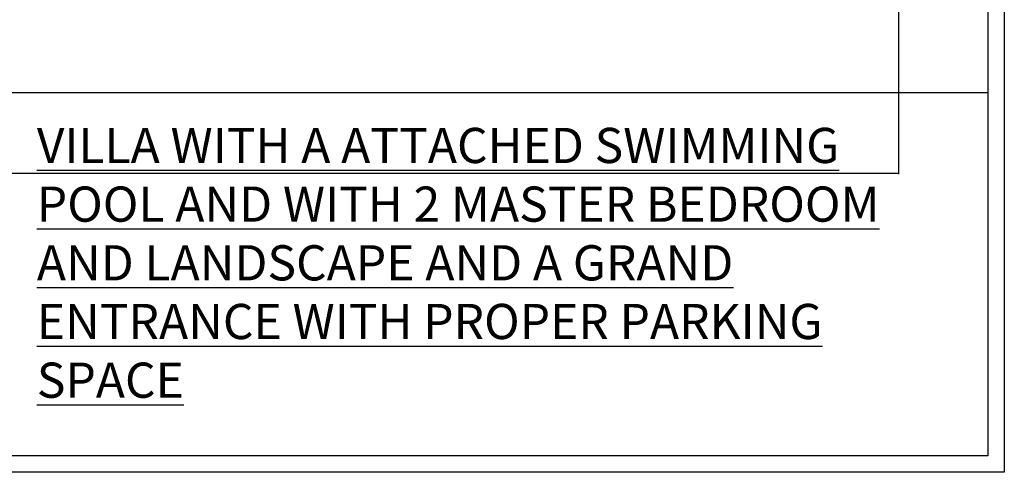
# Model space of a CAD drawing. Units: inches. Extents: x 84 to 1044, y -280 to 906.
# Tile 22 of 105: x 700 to 1027, y -280 to -129. Entities that reach past the tile are written whole.
import ezdxf

# ---------------------------------------------------------------- set-up
doc = ezdxf.new("R2010")
doc.units = ezdxf.units.IN
doc.layers.add('A-ANNO-DIMS', color=2, linetype='Continuous', lineweight=18)
doc.layers.add('A-ANNO-TTLB', color=7, linetype='Continuous', lineweight=25)
doc.styles.add('1-100DIM', font='txt', dxfattribs={"height": 0.3})
doc.styles.get("Standard").update_dxf_attribs({"font": 'arial.ttf'})
doc.dimstyles.get("Standard").update_dxf_attribs({"dimtxt": 0.18, "dimasz": 0.18, "dimexe": 0.18, "dimexo": 0.0625, "dimgap": 0.09, "dimtad": 0, "dimtih": 1, "dimtoh": 1, "dimdec": 4, "dimzin": 0, "dimdsep": 46, "dimtxsty": 'Standard', "dimcen": 0.09, "dimadec": 0, "dimazin": 0, "dimtfac": 1, "dimtdec": 4, "dimtofl": 0, "dimtmove": 0, "dimatfit": 3, "dimfxl": 1, "dimtolj": 1, "dimtzin": 0, "dimarcsym": 0})

# ---------------------------------------------------------------- blocks, each defined once
blk = doc.blocks.new('*D60')
at = {"layer": 'A-ANNO-DIMS', "color": 0, "lineweight": -2, "transparency": 16777216}
for p, q in [((134.18, -121.94), (134.18, -180.64)), ((992.07, -121.94), (992.07, -180.64)), ((134.36, -180.46), (562.73, -180.46)), ((991.89, -180.46), (563.52, -180.46))]:
    blk.add_line(p, q, dxfattribs=at)
at = {"layer": 'A-ANNO-DIMS', "color": 0, "transparency": 16777216}
for points in [[(134.36, -180.43), (134.36, -180.49), (134.18, -180.46)], [(991.89, -180.43), (991.89, -180.49), (992.07, -180.46)]]:
    blk.add_solid(points, dxfattribs=at)
at = {"layer": 'Defpoints', "color": 0, "transparency": 16777216}
for p in [(134.18, -121.88), (992.07, -121.88), (992.07, -180.46)]:
    blk.add_point(p, dxfattribs=at)
at = {"layer": 'A-ANNO-DIMS', "color": 0, "transparency": 16777216, "insert": (563.13, -180.46), "char_height": 0.18, "attachment_point": 5}
blk.add_mtext('\\A1;857.9', dxfattribs=at)

msp = doc.modelspace()

# ---------------------------------------------------------------- linework, layer by layer
at = {"layer": 'A-ANNO-TTLB'}
msp.add_line((106.576, -153.519), (1021.832, -153.519), dxfattribs=at)
for points in [[(101.1, 905.916), (1027.308, 905.916), (1027.308, -279.764), (101.1, -279.764)], [(106.576, 900.439), (1021.832, 900.439), (1021.832, -274.288), (106.576, -274.288)]]:
    msp.add_lwpolyline(points, close=True, dxfattribs=at)

# ---------------------------------------------------------------- texts
at = {"layer": 'A-ANNO-TTLB', "insert": (705.561, -165.274), "char_height": 11.700495, "attachment_point": 1, "style": '1-100DIM'}
msp.add_mtext_dynamic_manual_height_columns('{\\f@Malgun Gothic|b0|i0|c0|p34;\\LVILLA WITH A ATTACHED SWIMMING POOL AND WITH 2 MASTER BEDROOM AND LANDSCAPE AND A GRAND ENTRANCE WITH PROPER PARKING SPACE}', width=307.54906, gutter_width=24.488, heights=[0], dxfattribs=at)

# ---------------------------------------------------------------- dimensions: what is measured, and where the dimension line sits
at = {"layer": 'A-ANNO-DIMS'}
dim = msp.add_linear_dim(base=(992.074, -180.46), p1=(134.179, -121.88), p2=(992.074, -121.88), dimstyle='Standard', override={"dimdec": 1, "dimlfac": 1, "dimrnd": 0, "dimzin": 0, "dimdsep": 46, "dimlunit": 2}, dxfattribs=at)
dim.commit()
dim.dimension.update_dxf_attribs({"geometry": '*D60', "text_midpoint": (563.127, -180.46)})

doc.saveas('drawing.dxf')
